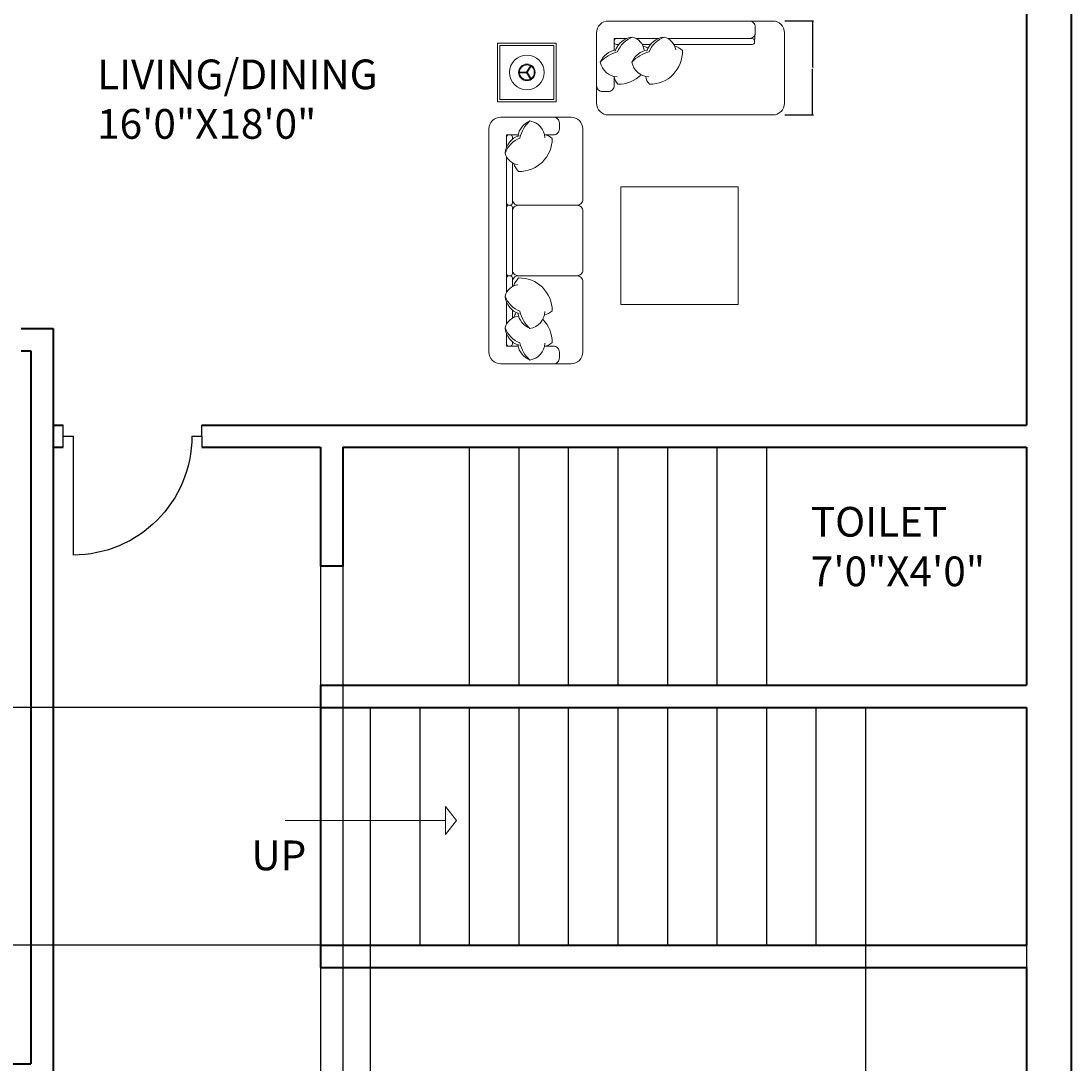
# Model space of a CAD drawing. Units: inches. Extents: x -19 to 419, y -828 to 43.
# Tile 7 of 9: x 198 to 410, y -574 to -364. Entities that reach past the tile are written whole.
import ezdxf

# ---------------------------------------------------------------- set-up
doc = ezdxf.new("R2010")
doc.units = ezdxf.units.IN
doc.header["$MEASUREMENT"] = 0
for name, color, linetype, lineweight in [('A-ANNO-DIMS', 2, 'Continuous', 18), ('A-ANNO-SYMB', 7, 'Continuous', 18), ('A-ANNO-TEXT', 7, 'Continuous', 18), ('A-AREA-IDEN', 7, 'Continuous', 25), ('A-DOOR', 3, 'Continuous', 25), ('A-FLOR-STRS', 7, 'Continuous', 25), ('A-FURN', 8, 'Continuous', 18), ('A-WALL', 7, 'Continuous', 40)]:
    doc.layers.add(name, color=color, linetype=linetype, lineweight=lineweight)
doc.styles.get("Standard").update_dxf_attribs({"font": 'arial.ttf'})
doc.dimstyles.get("Standard").update_dxf_attribs({"dimtxt": 0.18, "dimasz": 0.18, "dimexe": 0.18, "dimexo": 0.0625, "dimgap": 0.09, "dimtad": 0, "dimtih": 1, "dimtoh": 1, "dimdec": 0, "dimzin": 0, "dimdsep": 46, "dimlunit": 3, "dimtxsty": 'Standard', "dimcen": 0.09, "dimadec": 0, "dimazin": 0, "dimtfac": 1, "dimtdec": 0, "dimtofl": 0, "dimtmove": 0, "dimatfit": 3, "dimfxl": 1, "dimtolj": 1, "dimtzin": 0, "dimarcsym": 0})

# ---------------------------------------------------------------- blocks, each defined once
blk = doc.blocks.new('DAY BED1')
at = {"color": 0}
blk.add_line((0.3, 0.25), (0.225, 0.2549), dxfattribs=at)
blk.add_lwpolyline([(-0.3, 0, -0.414214), (-0.4, 0.1), (-0.4, 0.1, 0.317837), (-0.4, 0.1, -0.414214), (-0.4, 0.1), (-0.4, 0.1, 1.186185), (-0.4, 0.1, -0.414214), (-0.4, 0.1), (-0.4, 1.5, -0.414214), (-0.3, 1.6), (0.3, 1.6, -0.414214), (0.4, 1.5), (0.4, 0.1, -0.414214), (0.3, 0)], format="xyb", close=True, dxfattribs=at)
for points in [[(-0.0725, 1.45), (-0.15, 1.45, -0.414214), (-0.2, 1.5), (-0.2, 1.55, -0.414214), (-0.15, 1.6)], [(-0.0756, 1.4249, -0.356772), (0.0505, 1.5682, -0.249542), (0.1543, 1.4384, 9.61688)], [(0.0505, 1.5682, -0.14773), (0.1364, 1.422, -0.213343), (0.2624, 1.2931, -0.178662)], [(-0.0725, 1.4501, 0.165541), (-0.1386, 1.4192, 0.200231), (-0.0581, 1.2207, 0.121523)], [(0.1433, 1.4422, -0.306663), (0.2624, 1.2931, -0.30633), (0.1536, 1.1957, 0.872847)], [(0.25, 1.3448), (0.25, 1.45), (0.1517, 1.45, -0.414214)], [(0.2, 1.4118), (0.2, 1.43, -0.414214), (0.22, 1.45), (0.23, 1.45, -0.414214), (0.25, 1.43)], [(0.25, 1.43), (0.25, 1.3448, -0.414214)], [(-0.0756, 1.1556, -0.356772), (0.0505, 1.2988, -0.249542), (0.1543, 1.169, 9.61688)], [(0.0505, 1.2988, -0.14773), (0.1364, 1.1527, -0.213343), (0.2624, 1.0238, -0.178662)], [(0.25, 1.2616), (0.25, 1.0755, -0.414214)], [(-0.0725, 1.1808, 0.165541), (-0.1386, 1.1498, 0.425989), (0.1479, 0.869, 0.121523), (0.1873, 0.9357, -7.115464)], [(0.1433, 1.1729, -0.306663), (0.2624, 1.0238, -0.30633), (0.1536, 0.9263, 0.872847)], [(0.1678, 1.1631, 0.071865), (0.1873, 1.205, -7.115464)], [(0.2, 1.1425), (0.2, 1.2113, -0.414214)], [(0.25, 0.9923), (0.25, 0.2749, -0.414214), (0.23, 0.2549), (0.22, 0.2549, -0.414214), (0.2, 0.2749), (0.2, 0.9419, -0.414214)], [(0.25, 0.3775), (0.25, 0.3, 0.414214), (0.3, 0.25), (0.35, 0.25, 0.414214), (0.4, 0.3)]]:
    blk.add_lwpolyline(points, format="xyb", dxfattribs=at)
for points in [[(0.25, 1.0755), (0.25, 1.2616)], [(0.25, 0.3775), (0.25, 0.9923)]]:
    blk.add_lwpolyline(points, dxfattribs=at)
blk = doc.blocks.new('DOOR-24-PARTITION')
for p, q in [((2, 2.25), (2, 26.25)), ((0, 4.5), (0, 0)), ((28, 2.25), (28, 4.5)), ((0, 2.25), (2, 2.25)), ((26, 2.25), (28, 2.25)), ((28, 2.25), (28, 0))]:
    blk.add_line(p, q)
blk.add_arc((2, 2.25), 24, 0, 90)
blk = doc.blocks.new('*D43')
at = {"layer": 'A-ANNO-DIMS', "color": 0, "lineweight": -2, "transparency": 16777216}
for p, q in [((351.95, -363.66), (357.76, -363.66)), ((357.58, -363.84), (357.58, -372.97)), ((357.58, -382.45), (357.58, -373.33)), ((351.95, -382.63), (357.76, -382.63))]:
    blk.add_line(p, q, dxfattribs=at)
at = {"layer": 'A-ANNO-DIMS', "color": 0, "transparency": 16777216}
for points in [[(357.55, -363.84), (357.61, -363.84), (357.58, -363.66)], [(357.55, -382.45), (357.61, -382.45), (357.58, -382.63)]]:
    blk.add_solid(points, dxfattribs=at)
at = {"layer": 'Defpoints', "color": 0, "transparency": 16777216}
for p in [(351.89, -363.66), (357.58, -363.66), (351.89, -382.63)]:
    blk.add_point(p, dxfattribs=at)
at = {"layer": 'A-ANNO-DIMS', "color": 0, "transparency": 16777216, "insert": (357.58, -373.15), "char_height": 0.18, "attachment_point": 5}
blk.add_mtext('\\A1;1\'-7"', dxfattribs=at)
blk = doc.blocks.new('*D44')
at = {"layer": 'A-ANNO-DIMS', "color": 0, "lineweight": -2, "transparency": 16777216}
for p, q in [((258.18, -502.23), (-19.04, -502.23)), ((-18.86, -502.41), (-18.86, -526.05)), ((-18.86, -550.05), (-18.86, -526.42)), ((258.18, -550.23), (-19.04, -550.23))]:
    blk.add_line(p, q, dxfattribs=at)
at = {"layer": 'A-ANNO-DIMS', "color": 0, "transparency": 16777216}
for points in [[(-18.89, -502.41), (-18.83, -502.41), (-18.86, -502.23)], [(-18.89, -550.05), (-18.83, -550.05), (-18.86, -550.23)]]:
    blk.add_solid(points, dxfattribs=at)
at = {"layer": 'Defpoints', "color": 0, "transparency": 16777216}
for p in [(-18.86, -502.23), (258.24, -502.23), (258.24, -550.23)]:
    blk.add_point(p, dxfattribs=at)
at = {"layer": 'A-ANNO-DIMS', "color": 0, "transparency": 16777216, "insert": (-18.86, -526.23), "char_height": 0.18, "attachment_point": 5}
blk.add_mtext('\\A1;4\'-0"', dxfattribs=at)
blk = doc.blocks.new('*D45')
at = {"layer": 'A-ANNO-DIMS', "color": 0, "lineweight": -2, "transparency": 16777216}
for p, q in [((258.24, -550.3), (258.24, -827.51)), ((268.24, -550.3), (268.24, -827.51)), ((258.42, -827.33), (262.84, -827.33)), ((268.06, -827.33), (263.64, -827.33))]:
    blk.add_line(p, q, dxfattribs=at)
at = {"layer": 'A-ANNO-DIMS', "color": 0, "transparency": 16777216}
for points in [[(258.42, -827.3), (258.42, -827.36), (258.24, -827.33)], [(268.06, -827.3), (268.06, -827.36), (268.24, -827.33)]]:
    blk.add_solid(points, dxfattribs=at)
at = {"layer": 'Defpoints', "color": 0, "transparency": 16777216}
for p in [(258.24, -550.23), (268.24, -550.23), (268.24, -827.33)]:
    blk.add_point(p, dxfattribs=at)
at = {"layer": 'A-ANNO-DIMS', "color": 0, "transparency": 16777216, "insert": (263.24, -827.33), "char_height": 0.18, "attachment_point": 5}
blk.add_mtext('\\A1;0\'-10"', dxfattribs=at)
blk = doc.blocks.new('*D46')
at = {"layer": 'A-ANNO-DIMS', "color": 0, "lineweight": -2, "transparency": 16777216}
for p, q in [((368.24, -550.3), (368.24, -827.51)), ((400.74, -550.3), (400.74, -827.51)), ((368.42, -827.33), (383.95, -827.33)), ((400.56, -827.33), (385.03, -827.33))]:
    blk.add_line(p, q, dxfattribs=at)
at = {"layer": 'A-ANNO-DIMS', "color": 0, "transparency": 16777216}
for points in [[(368.42, -827.3), (368.42, -827.36), (368.24, -827.33)], [(400.56, -827.3), (400.56, -827.36), (400.74, -827.33)]]:
    blk.add_solid(points, dxfattribs=at)
at = {"layer": 'Defpoints', "color": 0, "transparency": 16777216}
for p in [(368.24, -550.23), (400.74, -550.23), (400.74, -827.33)]:
    blk.add_point(p, dxfattribs=at)
at = {"layer": 'A-ANNO-DIMS', "color": 0, "transparency": 16777216, "insert": (384.49, -827.33), "char_height": 0.18, "attachment_point": 5}
blk.add_mtext('\\A1;2\'-8 1/2"', dxfattribs=at)
blk = doc.blocks.new('*D48')
at = {"layer": 'A-ANNO-DIMS', "color": 0, "lineweight": -2, "transparency": 16777216}
for p, q in [((258.24, -473.8), (258.24, -827.51)), ((262.74, -473.8), (262.74, -827.51)), ((258.42, -827.33), (259.95, -827.33)), ((262.56, -827.33), (261.03, -827.33))]:
    blk.add_line(p, q, dxfattribs=at)
at = {"layer": 'A-ANNO-DIMS', "color": 0, "transparency": 16777216}
for points in [[(258.42, -827.3), (258.42, -827.36), (258.24, -827.33)], [(262.56, -827.3), (262.56, -827.36), (262.74, -827.33)]]:
    blk.add_solid(points, dxfattribs=at)
at = {"layer": 'Defpoints', "color": 0, "transparency": 16777216}
for p in [(258.24, -473.73), (262.74, -473.73), (262.74, -827.33)]:
    blk.add_point(p, dxfattribs=at)
at = {"layer": 'A-ANNO-DIMS', "color": 0, "transparency": 16777216, "insert": (260.49, -827.33), "char_height": 0.18, "attachment_point": 5}
blk.add_mtext('\\A1;0\'-4 1/2"', dxfattribs=at)

msp = doc.modelspace()

# ---------------------------------------------------------------- linework, layer by layer
at = {"layer": 'A-ANNO-SYMB'}
for p, q in [((283.47, -525.05), (283.47, -522.22)), ((283.47, -522.22), (285.64, -525.05)), ((251.09, -525.05), (283.47, -525.05)), ((283.47, -525.05), (283.47, -527.88)), ((283.47, -527.88), (285.64, -525.05))]:
    msp.add_line(p, q, dxfattribs=at)
at = {"layer": 'A-FLOR-STRS'}
for p, q in [((288.24, -449.73), (288.24, -497.73)), ((298.24, -449.73), (298.24, -497.73)), ((308.24, -449.73), (308.24, -497.73)), ((318.24, -449.73), (318.24, -497.73)), ((328.24, -449.73), (328.24, -497.73)), ((338.24, -449.73), (338.24, -497.73)), ((348.24, -449.73), (348.24, -497.73)), ((268.24, -502.23), (268.24, -550.23)), ((278.24, -502.23), (278.24, -550.23)), ((288.24, -502.23), (288.24, -550.23)), ((298.24, -502.23), (298.24, -550.23)), ((308.24, -502.23), (308.24, -550.23)), ((318.24, -502.23), (318.24, -550.23)), ((328.24, -502.23), (328.24, -550.23)), ((338.24, -502.23), (338.24, -550.23)), ((348.24, -502.23), (348.24, -550.23)), ((358.24, -502.23), (358.24, -550.23)), ((368.24, -502.23), (368.24, -550.23))]:
    msp.add_line(p, q, dxfattribs=at)
at = {"layer": 'A-FURN'}
for p, q in [((299.82, -374), (300.66, -372.56)), ((299.95, -374.08), (300.79, -372.63)), ((299.88, -373.97), (298.21, -373.97)), ((299.88, -374.12), (298.21, -374.12)), ((299.82, -374.08), (300.66, -375.53)), ((299.95, -374), (300.79, -375.45))]:
    msp.add_line(p, q, dxfattribs=at)
at = {"layer": 'A-FURN', "ltscale": 0.03}
for points in [[(305.81, -368.11), (305.81, -379.97), (293.96, -379.97), (293.96, -368.11)], [(342.57, -420.87), (342.57, -397.16), (318.85, -397.16), (318.85, -420.87)]]:
    msp.add_lwpolyline(points, close=True, dxfattribs=at)
at = {"layer": 'A-FURN'}
msp.add_lwpolyline([(305.34, -379.49), (305.34, -368.59), (294.43, -368.59), (294.43, -379.49)], close=True, dxfattribs=at)
at = {"layer": 'A-FURN', "ltscale": 0.03}
msp.add_lwpolyline([(308.81, -383.08, -0.414214), (311.18, -385.45), (311.18, -399.68, -0.414214), (309.99, -400.87, -0.414214), (311.18, -402.05), (311.18, -413.91, -0.414214), (309.99, -415.09, -0.414214), (311.18, -416.28), (311.18, -430.51, -0.414214), (308.81, -432.88), (294.58, -432.88, -0.414214), (292.21, -430.51), (292.21, -385.45, -0.414214), (294.58, -383.08)], format="xyb", close=True, dxfattribs=at)
at = {"layer": 'A-FURN'}
for points in [[(305.25, -383.08, -0.414214), (306.44, -384.27), (306.44, -385.45, -0.414214), (305.25, -386.64), (303.42, -386.64)], [(300.5, -383.84, 0.14773), (298.46, -387.3, 0.213343), (295.47, -390.36, 0.178662)], [(303.49, -387.23, 0.356772), (300.5, -383.84, 0.249542), (298.04, -386.92, -9.61688)], [(298.3, -386.82, 0.306663), (295.47, -390.36, 0.30633), (298.05, -392.67, -0.872847)], [(296.95, -387.54), (296.95, -387.11, 0.414214), (296.48, -386.64), (296.24, -386.64, 0.414214), (295.77, -387.11)], [(295.77, -387.11), (295.77, -389.13, 0.414214)], [(303.42, -386.64, -0.165541), (304.98, -387.37, -0.425989), (298.19, -394.03, -0.121523), (297.25, -392.45, 7.115464)], [(295.77, -391.11), (295.77, -400.39, 0.414214), (296.24, -400.87), (296.48, -400.87, 0.414214), (296.95, -400.39), (296.95, -392.3, 0.414214)], [(296.95, -399.68, 0.414214), (298.14, -400.87), (309.99, -400.87, 0.414214)], [(296.95, -402.05, -0.414214), (298.14, -400.87)], [(295.77, -418.47), (295.77, -415.57, -0.414214), (296.24, -415.09), (296.48, -415.09, -0.414214), (296.95, -415.57), (296.95, -417.27, -0.414214)], [(296.95, -413.91, 0.414214), (298.14, -415.09)], [(296.95, -416.28, -0.414214), (298.14, -415.09), (309.99, -415.09, -0.414214)], [(298.3, -422.75, -0.306663), (295.47, -419.21, -0.30633), (298.05, -416.9, 0.872847)], [(303.42, -422.94, 0.165541), (304.98, -422.2, 0.425989), (298.19, -415.54, 0.121523), (297.25, -417.13, -7.115464)], [(300.5, -425.74, -0.14773), (298.46, -422.27, -0.213343), (295.47, -419.21, -0.178662)], [(295.77, -424.85), (295.77, -420.44, -0.414214)], [(298.3, -429.14, -0.306663), (295.47, -425.6, -0.30633), (298.05, -423.29, 0.872847)], [(296.95, -422.03), (296.95, -423.66, -0.414214)], [(297.72, -422.52, 0.071865), (297.25, -423.51, -7.115464)], [(303.49, -422.34, -0.356772), (300.5, -425.74, -0.249542), (298.04, -422.66, 9.61688)], [(303.42, -429.32, 0.165541), (304.98, -428.59, 0.200231), (303.07, -423.88, 0.121523)], [(300.5, -432.12, -0.14773), (298.46, -428.66, -0.213343), (295.47, -425.6, -0.178662)], [(295.77, -426.83), (295.77, -429.32), (298.1, -429.32, -0.414214)], [(295.77, -428.85), (295.77, -426.83, -0.414214)], [(296.95, -428.42), (296.95, -428.85, -0.414214), (296.48, -429.32), (296.24, -429.32, -0.414214), (295.77, -428.85)], [(303.49, -428.73, -0.356772), (300.5, -432.12, -0.249542), (298.04, -429.04, 9.61688)], [(303.42, -429.32), (305.25, -429.32, -0.414214), (306.44, -430.51), (306.44, -431.69, -0.414214), (305.25, -432.88)]]:
    msp.add_lwpolyline(points, format="xyb", dxfattribs=at)
for points in [[(298.1, -386.64), (295.77, -386.64), (295.77, -389.13)], [(295.77, -391.11), (295.77, -418.47)], [(295.77, -420.44), (295.77, -424.85)]]:
    msp.add_lwpolyline(points, dxfattribs=at)
msp.add_lwpolyline([(295.77, -414.62), (295.77, -401.34, -0.414214), (296.24, -400.87), (296.48, -400.87, -0.414214), (296.95, -401.34), (296.95, -414.62, -0.414214), (296.48, -415.09), (296.24, -415.09, -0.414214)], format="xyb", close=True, dxfattribs=at)
for radius in [3.5, 1.67, 1.5]:
    msp.add_circle((299.88, -374.04), radius, dxfattribs=at)
at = {"layer": 'A-WALL'}
for p, q in [((400.74, -259.23), (400.74, -445.23)), ((409.74, -259.23), (409.74, -785.73)), ((197.74, -425.73), (204.24, -425.73)), ((204.24, -425.73), (204.24, -430.23)), ((197.74, -430.23), (199.74, -430.23)), ((199.74, -430.23), (199.74, -574.23)), ((204.24, -430.23), (204.24, -644.73)), ((204.24, -445.23), (206.24, -445.23)), ((234.24, -445.23), (400.74, -445.23)), ((204.24, -449.73), (206.24, -449.73)), ((234.24, -449.73), (258.24, -449.73)), ((258.24, -449.73), (258.24, -473.73)), ((262.74, -449.73), (262.74, -473.73)), ((262.74, -449.73), (312.24, -449.73)), ((312.24, -449.73), (316.74, -449.73)), ((316.74, -449.73), (400.74, -449.73)), ((400.74, -449.73), (400.74, -497.73)), ((262.74, -473.73), (258.24, -473.73)), ((258.24, -497.73), (400.74, -497.73)), ((258.24, -497.73), (258.24, -554.73)), ((258.24, -502.23), (400.74, -502.23)), ((400.74, -502.23), (400.74, -550.23)), ((258.24, -550.23), (400.74, -550.23)), ((258.24, -554.73), (400.74, -554.73)), ((400.74, -554.73), (400.74, -674.73)), ((31.74, -574.23), (199.74, -574.23))]:
    msp.add_line(p, q, dxfattribs=at)

# ---------------------------------------------------------------- block references
at = {"layer": 'A-DOOR', "extrusion": (0, 0, -1), "zscale": -1, "rotation": 180}
msp.add_blockref('DOOR-24-PARTITION', (-206.24, -445.23), dxfattribs=at)
at = {"layer": 'A-FURN', "ltscale": 0.03, "xscale": 23.71147996292152, "yscale": 23.71147996292152, "zscale": 23.71147996292152, "rotation": 90}
msp.add_blockref('DAY BED1', (351.89, -373.15), dxfattribs=at)

# ---------------------------------------------------------------- texts
at = {"layer": 'A-ANNO-TEXT', "insert": (244.26, -529.11), "char_height": 6, "attachment_point": 1}
msp.add_mtext('UP', dxfattribs=at)
at = {"layer": 'A-AREA-IDEN', "char_height": 6, "attachment_point": 1}
for s, insert in [('LIVING/DINING\\P16\'0"X18\'0"', (213.11, -371.44)), ('TOILET\\P7\'0"X4\'0"', (357.21, -461.77))]:
    msp.add_mtext(s, dxfattribs=dict(at, insert=insert))

# ---------------------------------------------------------------- dimensions: what is measured, and where the dimension line sits
at = {"layer": 'A-ANNO-DIMS'}
for base, p1, p2, picture, middle in [((357.58, -363.66), (351.89, -382.63), (351.89, -363.66), '*D43', (357.58, -373.15)), ((-18.86, -502.23), (258.24, -550.23), (258.24, -502.23), '*D44', (-18.86, -526.23))]:
    dim = msp.add_linear_dim(base=base, p1=p1, p2=p2, angle=90, dimstyle='Standard', override={"dimdec": 1, "dimlfac": 1, "dimrnd": 0, "dimzin": 1, "dimdsep": 46, "dimlunit": 4, "dimfrac": 2}, dxfattribs=at)
    dim.commit()
    dim.dimension.update_dxf_attribs({"geometry": picture, "text_midpoint": middle})
for base, p1, p2, picture, middle in [((262.74, -827.33), (258.24, -473.73), (262.74, -473.73), '*D48', (260.49, -827.33)), ((268.24, -827.33), (258.24, -550.23), (268.24, -550.23), '*D45', (263.24, -827.33)), ((400.74, -827.33), (368.24, -550.23), (400.74, -550.23), '*D46', (384.49, -827.33))]:
    dim = msp.add_linear_dim(base=base, p1=p1, p2=p2, dimstyle='Standard', override={"dimdec": 1, "dimlfac": 1, "dimrnd": 0, "dimzin": 1, "dimdsep": 46, "dimlunit": 4, "dimfrac": 2}, dxfattribs=at)
    dim.commit()
    dim.dimension.update_dxf_attribs({"geometry": picture, "text_midpoint": middle})

doc.saveas('drawing.dxf')
